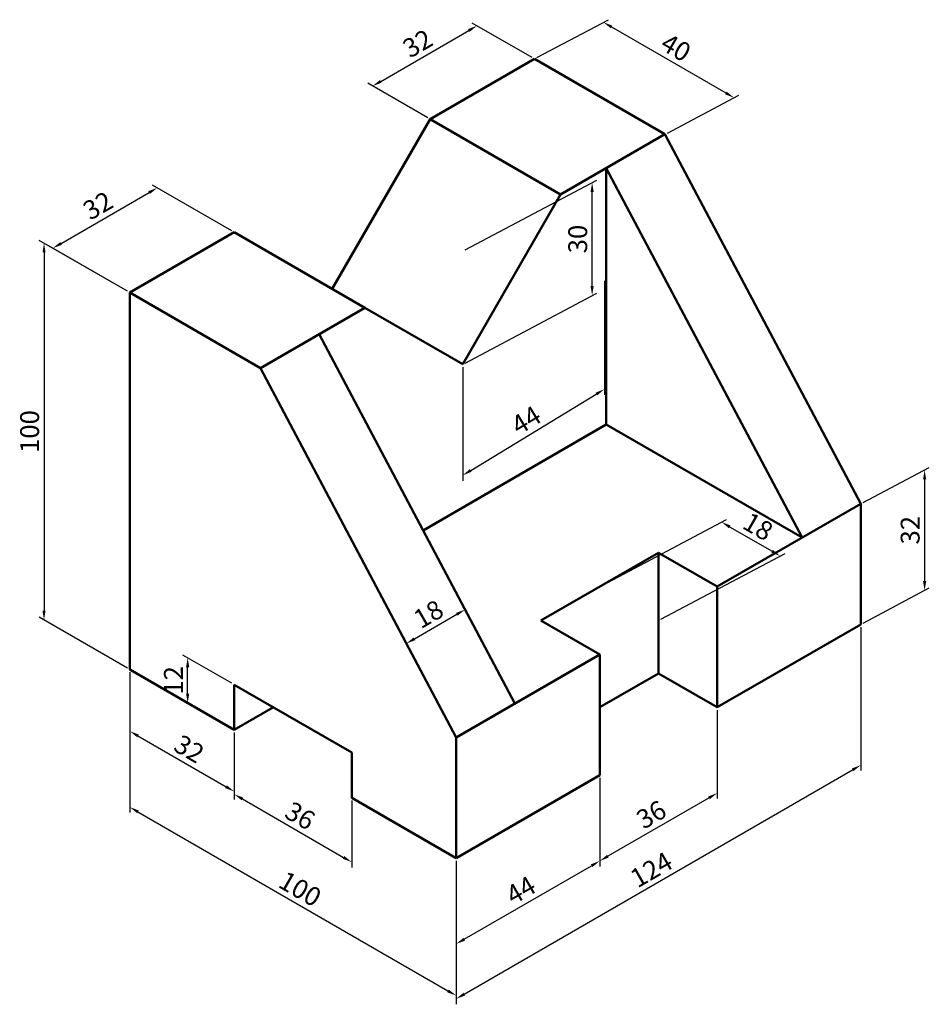
# Model space of a CAD drawing. Units: millimetres. Extents: x 91 to 333, y -17 to 244.
import ezdxf

# ---------------------------------------------------------------- set-up
doc = ezdxf.new("R2010")
doc.units = ezdxf.units.MM
doc.layers.add('M-DIMS', color=2, linetype='Continuous', lineweight=25)
doc.layers.add('M-OUTL', color=7, linetype='Continuous', lineweight=50)
doc.styles.get("Standard").update_dxf_attribs({"font": 'arial.ttf'})
doc.dimstyles.new('ISO-25', dxfattribs={"dimtxt": 5, "dimasz": 2.5, "dimexe": 1.25, "dimexo": 0.625, "dimtad": 1, "dimtxsty": 'Standard', "dimcen": 2.5, "dimadec": 0, "dimazin": 0, "dimtfac": 1, "dimtmove": 0, "dimatfit": 3, "dimfxl": 1, "dimarcsym": 0})

# ---------------------------------------------------------------- blocks, each defined once
blk = doc.blocks.new('*D1')
at = {"layer": 'Defpoints', "color": 0, "transparency": 16777216}
for p in [(127.79, 199.74), (148.21, 187.94), (120.5, 171.94)]:
    blk.add_point(p, dxfattribs=at)
at = {"layer": 'M-DIMS', "color": 0, "lineweight": -2, "transparency": 16777216}
for p, q in [((147.59, 188.3), (126.54, 200.46)), ((102.24, 184.99), (125.62, 198.49)), ((119.88, 172.3), (98.82, 184.46))]:
    blk.add_line(p, q, dxfattribs=at)
at = {"layer": 'M-DIMS', "color": 0, "transparency": 16777216}
for points in [[(125.41, 198.85), (125.83, 198.13), (127.79, 199.74)], [(102.03, 185.35), (102.45, 184.63), (100.07, 183.74)]]:
    blk.add_solid(points, dxfattribs=at)
at = {"layer": 'M-DIMS', "color": 0, "transparency": 16777216, "insert": (112.34, 194.49), "char_height": 5, "attachment_point": 5, "rotation": 30}
blk.add_mtext('32', dxfattribs=at)
blk = doc.blocks.new('*D2')
at = {"layer": 'Defpoints', "color": 0, "transparency": 16777216}
for p in [(227.89, 233.94), (280.85, 223.66), (262.53, 213.94)]:
    blk.add_point(p, dxfattribs=at)
at = {"layer": 'M-DIMS', "color": 0, "lineweight": -2, "transparency": 16777216}
for p, q in [((228.54, 234.29), (247.51, 244.35)), ((248.37, 242.41), (278.68, 224.91)), ((263.18, 214.29), (282.15, 224.35))]:
    blk.add_line(p, q, dxfattribs=at)
at = {"layer": 'M-DIMS', "color": 0, "transparency": 16777216}
for points in [[(248.58, 242.77), (248.17, 242.05), (246.21, 243.66)], [(278.89, 225.27), (278.48, 224.55), (280.85, 223.66)]]:
    blk.add_solid(points, dxfattribs=at)
at = {"layer": 'M-DIMS', "color": 0, "transparency": 16777216, "insert": (265.12, 236.41), "char_height": 5, "attachment_point": 5, "rotation": 330}
blk.add_mtext('40', dxfattribs=at)
blk = doc.blocks.new('*D3')
at = {"layer": 'Defpoints', "color": 0, "transparency": 16777216}
for p in [(120.5, 171.94), (97.73, 85.09), (120.5, 71.94)]:
    blk.add_point(p, dxfattribs=at)
at = {"layer": 'M-DIMS', "color": 0, "lineweight": -2, "transparency": 16777216}
for p, q in [((119.88, 172.3), (96.48, 185.81)), ((97.73, 182.59), (97.73, 87.59)), ((119.88, 72.3), (96.48, 85.81))]:
    blk.add_line(p, q, dxfattribs=at)
at = {"layer": 'M-DIMS', "color": 0, "transparency": 16777216}
for points in [[(97.32, 182.59), (98.15, 182.59), (97.73, 185.09)], [(97.32, 87.59), (98.15, 87.59), (97.73, 85.09)]]:
    blk.add_solid(points, dxfattribs=at)
at = {"layer": 'M-DIMS', "color": 0, "transparency": 16777216, "insert": (94.56, 135.09), "char_height": 5, "attachment_point": 5, "rotation": 90}
blk.add_mtext('100', dxfattribs=at)
blk = doc.blocks.new('*D4')
at = {"layer": 'Defpoints', "color": 0, "transparency": 16777216}
for p in [(209.48, 87.87), (222.69, 62.94), (207.1, 53.94)]:
    blk.add_point(p, dxfattribs=at)
at = {"layer": 'M-DIMS', "color": 0, "lineweight": -2, "transparency": 16777216}
for p, q in [((222.4, 63.5), (208.89, 88.97)), ((196.05, 80.12), (207.31, 86.62)), ((206.81, 54.5), (193.3, 79.97))]:
    blk.add_line(p, q, dxfattribs=at)
at = {"layer": 'M-DIMS', "color": 0, "transparency": 16777216}
for points in [[(207.1, 86.98), (207.52, 86.26), (209.48, 87.87)], [(195.85, 80.48), (196.26, 79.76), (193.89, 78.87)]]:
    blk.add_solid(points, dxfattribs=at)
at = {"layer": 'M-DIMS', "color": 0, "transparency": 16777216, "insert": (200.09, 86.12), "char_height": 5, "attachment_point": 5, "rotation": 30}
blk.add_mtext('18', dxfattribs=at)
blk = doc.blocks.new('*D5')
at = {"layer": 'Defpoints', "color": 0, "transparency": 16777216}
for p in [(120.5, 71.94), (148.21, 55.94), (148.21, 39.61)]:
    blk.add_point(p, dxfattribs=at)
at = {"layer": 'M-DIMS', "color": 0, "lineweight": -2, "transparency": 16777216}
for p, q in [((120.5, 71.22), (120.5, 54.17)), ((148.21, 55.22), (148.21, 38.17)), ((122.67, 54.36), (146.05, 40.86))]:
    blk.add_line(p, q, dxfattribs=at)
at = {"layer": 'M-DIMS', "color": 0, "transparency": 16777216}
for points in [[(122.87, 54.72), (122.46, 54), (120.5, 55.61)], [(146.26, 41.22), (145.84, 40.5), (148.21, 39.61)]]:
    blk.add_solid(points, dxfattribs=at)
at = {"layer": 'M-DIMS', "color": 0, "transparency": 16777216, "insert": (135.95, 50.36), "char_height": 5, "attachment_point": 5, "rotation": 330}
blk.add_mtext('32', dxfattribs=at)
blk = doc.blocks.new('*D6')
at = {"layer": 'Defpoints', "color": 0, "transparency": 16777216}
for p in [(135.85, 75.08), (148.21, 67.94), (148.21, 55.94)]:
    blk.add_point(p, dxfattribs=at)
at = {"layer": 'M-DIMS', "color": 0, "lineweight": -2, "transparency": 16777216}
for p, q in [((147.59, 68.3), (134.6, 75.8)), ((135.85, 65.58), (135.85, 72.58)), ((147.59, 56.3), (134.6, 63.8))]:
    blk.add_line(p, q, dxfattribs=at)
at = {"layer": 'M-DIMS', "color": 0, "transparency": 16777216}
for points in [[(135.44, 72.58), (136.27, 72.58), (135.85, 75.08)], [(135.44, 65.58), (136.27, 65.58), (135.85, 63.08)]]:
    blk.add_solid(points, dxfattribs=at)
at = {"layer": 'M-DIMS', "color": 0, "transparency": 16777216, "insert": (132.72, 69.08), "char_height": 5, "attachment_point": 5, "rotation": 90}
blk.add_mtext('12', dxfattribs=at)
blk = doc.blocks.new('*D7')
at = {"layer": 'Defpoints', "color": 0, "transparency": 16777216}
for p in [(148.21, 55.94), (179.39, 37.94), (179.39, 20.88)]:
    blk.add_point(p, dxfattribs=at)
at = {"layer": 'M-DIMS', "color": 0, "lineweight": -2, "transparency": 16777216}
for p, q in [((148.21, 55.22), (148.21, 37.44)), ((150.38, 37.63), (177.23, 22.13)), ((179.39, 37.22), (179.39, 19.44))]:
    blk.add_line(p, q, dxfattribs=at)
at = {"layer": 'M-DIMS', "color": 0, "transparency": 16777216}
for points in [[(150.59, 37.99), (150.17, 37.27), (148.21, 38.88)], [(177.43, 22.49), (177.02, 21.77), (179.39, 20.88)]]:
    blk.add_solid(points, dxfattribs=at)
at = {"layer": 'M-DIMS', "color": 0, "transparency": 16777216, "insert": (165.39, 32.63), "char_height": 5, "attachment_point": 5, "rotation": 330}
blk.add_mtext('36', dxfattribs=at)
blk = doc.blocks.new('*D8')
at = {"layer": 'Defpoints', "color": 0, "transparency": 16777216}
for p in [(120.5, 71.94), (207.1, 21.94), (207.1, -14.54)]:
    blk.add_point(p, dxfattribs=at)
at = {"layer": 'M-DIMS', "color": 0, "lineweight": -2, "transparency": 16777216}
for p, q in [((120.5, 71.22), (120.5, 34.01)), ((122.67, 34.21), (204.94, -13.29)), ((207.1, 21.22), (207.1, -15.99))]:
    blk.add_line(p, q, dxfattribs=at)
at = {"layer": 'M-DIMS', "color": 0, "transparency": 16777216}
for points in [[(122.87, 34.57), (122.46, 33.85), (120.5, 35.46)], [(205.15, -12.93), (204.73, -13.65), (207.1, -14.54)]]:
    blk.add_solid(points, dxfattribs=at)
at = {"layer": 'M-DIMS', "color": 0, "transparency": 16777216, "insert": (165.39, 13.21), "char_height": 5, "attachment_point": 5, "rotation": 330}
blk.add_mtext('100', dxfattribs=at)
blk = doc.blocks.new('*D9')
at = {"layer": 'Defpoints', "color": 0, "transparency": 16777216}
for p in [(245.21, 43.94), (207.1, 21.94), (245.21, 21.17)]:
    blk.add_point(p, dxfattribs=at)
at = {"layer": 'M-DIMS', "color": 0, "lineweight": -2, "transparency": 16777216}
for p, q in [((245.21, 43.22), (245.21, 19.73)), ((207.1, 21.22), (207.1, -2.27)), ((209.27, 0.42), (243.04, 19.92))]:
    blk.add_line(p, q, dxfattribs=at)
at = {"layer": 'M-DIMS', "color": 0, "transparency": 16777216}
for points in [[(242.84, 20.28), (243.25, 19.56), (245.21, 21.17)], [(209.06, 0.78), (209.48, 0.06), (207.1, -0.83)]]:
    blk.add_solid(points, dxfattribs=at)
at = {"layer": 'M-DIMS', "color": 0, "transparency": 16777216, "insert": (224.59, 12.88), "char_height": 5, "attachment_point": 5, "rotation": 30}
blk.add_mtext('44', dxfattribs=at)
blk = doc.blocks.new('*D10')
at = {"layer": 'Defpoints', "color": 0, "transparency": 16777216}
for p in [(276.39, 61.94), (245.21, 43.94), (245.21, 21.18)]:
    blk.add_point(p, dxfattribs=at)
at = {"layer": 'M-DIMS', "color": 0, "lineweight": -2, "transparency": 16777216}
for p, q in [((276.39, 61.22), (276.39, 37.74)), ((245.21, 43.22), (245.21, 19.74)), ((274.22, 37.93), (247.37, 22.43))]:
    blk.add_line(p, q, dxfattribs=at)
at = {"layer": 'M-DIMS', "color": 0, "transparency": 16777216}
for points in [[(274.01, 38.29), (274.43, 37.57), (276.39, 39.18)], [(247.17, 22.79), (247.58, 22.07), (245.21, 21.18)]]:
    blk.add_solid(points, dxfattribs=at)
at = {"layer": 'M-DIMS', "color": 0, "transparency": 16777216, "insert": (259.21, 32.94), "char_height": 5, "attachment_point": 5, "rotation": 30}
blk.add_mtext('36', dxfattribs=at)
blk = doc.blocks.new('*D11')
at = {"layer": 'Defpoints', "color": 0, "transparency": 16777216}
for p in [(314.49, 83.94), (314.49, 46.6), (207.1, 21.94)]:
    blk.add_point(p, dxfattribs=at)
at = {"layer": 'M-DIMS', "color": 0, "lineweight": -2, "transparency": 16777216}
for p, q in [((314.49, 83.22), (314.49, 45.15)), ((209.27, -14.15), (312.33, 45.35)), ((207.1, 21.22), (207.1, -16.85))]:
    blk.add_line(p, q, dxfattribs=at)
at = {"layer": 'M-DIMS', "color": 0, "transparency": 16777216}
for points in [[(312.12, 45.71), (312.53, 44.99), (314.49, 46.6)], [(209.06, -13.79), (209.48, -14.51), (207.1, -15.4)]]:
    blk.add_solid(points, dxfattribs=at)
at = {"layer": 'M-DIMS', "color": 0, "transparency": 16777216, "insert": (259.23, 18.31), "char_height": 5, "attachment_point": 5, "rotation": 30}
blk.add_mtext('124', dxfattribs=at)
blk = doc.blocks.new('*D12')
at = {"layer": 'Defpoints', "color": 0, "transparency": 16777216}
for p in [(314.49, 115.94), (331.43, 92.92), (314.49, 83.94)]:
    blk.add_point(p, dxfattribs=at)
at = {"layer": 'M-DIMS', "color": 0, "lineweight": -2, "transparency": 16777216}
for p, q in [((315.12, 116.27), (332.68, 125.59)), ((331.43, 122.42), (331.43, 95.42)), ((315.12, 84.27), (332.68, 93.59))]:
    blk.add_line(p, q, dxfattribs=at)
at = {"layer": 'M-DIMS', "color": 0, "transparency": 16777216}
for points in [[(331.01, 122.42), (331.85, 122.42), (331.43, 124.92)], [(331.01, 95.42), (331.85, 95.42), (331.43, 92.92)]]:
    blk.add_solid(points, dxfattribs=at)
at = {"layer": 'M-DIMS', "color": 0, "transparency": 16777216, "insert": (328.25, 108.92), "char_height": 5, "attachment_point": 5, "rotation": 90}
blk.add_mtext('32', dxfattribs=at)
blk = doc.blocks.new('*D13')
at = {"layer": 'Defpoints', "color": 0, "transparency": 16777216}
for p in [(293.11, 102.08), (245.21, 93.94), (260.8, 84.94)]:
    blk.add_point(p, dxfattribs=at)
at = {"layer": 'M-DIMS', "color": 0, "lineweight": -2, "transparency": 16777216}
for p, q in [((245.86, 94.29), (278.83, 111.77)), ((279.69, 109.83), (290.95, 103.33)), ((261.45, 85.29), (294.42, 102.77))]:
    blk.add_line(p, q, dxfattribs=at)
at = {"layer": 'M-DIMS', "color": 0, "transparency": 16777216}
for points in [[(279.9, 110.19), (279.48, 109.47), (277.53, 111.08)], [(291.16, 103.69), (290.74, 102.97), (293.11, 102.08)]]:
    blk.add_solid(points, dxfattribs=at)
at = {"layer": 'M-DIMS', "color": 0, "transparency": 16777216, "insert": (286.91, 109.33), "char_height": 5, "attachment_point": 5, "rotation": 330}
blk.add_mtext('18', dxfattribs=at)
blk = doc.blocks.new('*D14')
at = {"layer": 'Defpoints', "color": 0, "transparency": 16777216}
for p in [(243.2, 201.16), (208.84, 182.94), (208.84, 152.94)]:
    blk.add_point(p, dxfattribs=at)
at = {"layer": 'M-DIMS', "color": 0, "lineweight": -2, "transparency": 16777216}
for p, q in [((209.46, 183.27), (244.45, 201.82)), ((243.2, 173.66), (243.2, 198.66)), ((209.46, 153.27), (244.45, 171.82))]:
    blk.add_line(p, q, dxfattribs=at)
at = {"layer": 'M-DIMS', "color": 0, "transparency": 16777216}
for points in [[(242.78, 198.66), (243.61, 198.66), (243.2, 201.16)], [(242.78, 173.66), (243.61, 173.66), (243.2, 171.16)]]:
    blk.add_solid(points, dxfattribs=at)
at = {"layer": 'M-DIMS', "color": 0, "transparency": 16777216, "insert": (240.02, 186.16), "char_height": 5, "attachment_point": 5, "rotation": 90}
blk.add_mtext('30', dxfattribs=at)
blk = doc.blocks.new('*D15')
at = {"layer": 'Defpoints', "color": 0, "transparency": 16777216}
for p in [(212.65, 242.74), (227.89, 233.94), (200.18, 217.94)]:
    blk.add_point(p, dxfattribs=at)
at = {"layer": 'M-DIMS', "color": 0, "lineweight": -2, "transparency": 16777216}
for p, q in [((227.26, 234.3), (211.4, 243.47)), ((187.1, 227.99), (210.48, 241.49)), ((199.55, 218.3), (183.68, 227.47))]:
    blk.add_line(p, q, dxfattribs=at)
at = {"layer": 'M-DIMS', "color": 0, "transparency": 16777216}
for points in [[(210.27, 241.85), (210.69, 241.13), (212.65, 242.74)], [(186.89, 228.35), (187.31, 227.63), (184.93, 226.74)]]:
    blk.add_solid(points, dxfattribs=at)
at = {"layer": 'M-DIMS', "color": 0, "transparency": 16777216, "insert": (197.2, 237.5), "char_height": 5, "attachment_point": 5, "rotation": 30}
blk.add_mtext('32', dxfattribs=at)
blk = doc.blocks.new('*D16')
at = {"layer": 'Defpoints', "color": 0, "transparency": 16777216}
for p in [(246.44, 175.8), (208.84, 152.94), (246.44, 146.32)]:
    blk.add_point(p, dxfattribs=at)
at = {"layer": 'M-DIMS', "color": 0, "lineweight": -2, "transparency": 16777216}
for p, q in [((246.44, 175.07), (246.44, 144.86)), ((208.84, 152.21), (208.84, 122.01)), ((210.97, 124.77), (244.3, 145.02))]:
    blk.add_line(p, q, dxfattribs=at)
at = {"layer": 'M-DIMS', "color": 0, "transparency": 16777216}
for points in [[(244.08, 145.38), (244.52, 144.67), (246.44, 146.32)], [(210.76, 125.12), (211.19, 124.41), (208.84, 123.47)]]:
    blk.add_solid(points, dxfattribs=at)
at = {"layer": 'M-DIMS', "color": 0, "transparency": 16777216, "insert": (226.01, 137.57), "char_height": 5, "attachment_point": 5, "rotation": 31.2909}
blk.add_mtext('44', dxfattribs=at)

msp = doc.modelspace()

# ---------------------------------------------------------------- linework, layer by layer
at = {"layer": 'M-OUTL'}
for p, q in [((200.175, 217.944), (227.888, 233.944)), ((227.888, 233.944), (262.529, 213.944)), ((174.195, 172.944), (200.175, 217.944)), ((200.175, 217.944), (234.816, 197.944)), ((262.529, 213.944), (234.816, 197.944)), ((262.529, 213.944), (314.491, 115.944)), ((246.941, 204.944), (298.902, 106.944)), ((246.941, 204.944), (246.941, 136.944)), ((208.836, 152.944), (234.816, 197.944)), ((148.214, 187.944), (120.501, 171.944)), ((182.855, 167.944), (148.214, 187.944)), ((120.501, 71.944), (120.501, 171.944)), ((120.501, 171.944), (155.142, 151.944)), ((155.142, 151.944), (182.855, 167.944)), ((208.836, 152.944), (182.855, 167.944)), ((170.731, 160.944), (222.692, 62.944)), ((155.142, 151.944), (207.104, 53.944)), ((246.941, 136.944), (198.335, 108.881)), ((298.902, 106.944), (246.941, 136.944)), ((276.386, 93.944), (314.491, 115.944)), ((314.491, 115.944), (314.491, 83.944)), ((229.62, 84.944), (260.797, 102.944)), ((276.386, 93.944), (260.797, 102.944)), ((260.797, 70.944), (260.797, 102.944)), ((276.386, 61.944), (276.386, 93.944)), ((245.209, 75.944), (229.62, 84.944)), ((314.491, 83.944), (276.386, 61.944)), ((207.104, 53.944), (245.209, 75.944)), ((245.209, 75.944), (245.209, 43.944)), ((120.501, 71.944), (148.214, 55.944)), ((245.209, 61.944), (260.797, 70.944)), ((276.386, 61.944), (260.797, 70.944)), ((148.214, 55.944), (148.214, 67.944)), ((148.214, 67.944), (179.391, 49.944)), ((148.214, 55.944), (158.606, 61.944)), ((207.104, 21.944), (207.104, 53.944)), ((179.391, 49.944), (179.391, 37.944)), ((245.209, 43.944), (207.104, 21.944)), ((179.391, 37.944), (207.104, 21.944))]:
    msp.add_line(p, q, dxfattribs=at)

# ---------------------------------------------------------------- dimensions: what is measured, and where the dimension line sits
at = {"layer": 'M-DIMS'}
for p1, p2, distance, picture, middle in [((200.175, 217.944), (227.888, 233.944), 15.242, '*D15', (197.2, 237.497)), ((227.888, 233.944), (262.529, 213.944), 17.573, '*D2', (265.118, 236.41)), ((208.836, 152.944), (208.836, 182.944), -34.36, '*D14', (240.016, 186.162)), ((120.501, 171.944), (148.214, 187.944), 20.428, '*D1', (112.339, 194.491)), ((120.501, 171.944), (120.501, 71.944), -22.768, '*D3', (94.555, 135.089)), ((208.836, 152.944), (246.436, 175.796), -25.187, '*D16', (226.013, 137.566)), ((314.491, 115.944), (314.491, 83.944), 16.938, '*D12', (328.249, 108.924)), ((245.209, 93.944), (260.797, 84.944), 30.998, '*D13', (286.909, 109.331)), ((207.104, 53.944), (222.692, 62.944), 28.193, '*D4', (200.094, 86.12)), ((207.104, 21.944), (314.491, 83.944), -32.344, '*D11', (259.23, 18.311)), ((148.214, 55.944), (148.214, 67.944), 12.36, '*D6', (132.718, 69.08)), ((120.501, 71.944), (148.214, 55.944), -14.146, '*D5', (135.947, 50.362)), ((120.501, 71.944), (207.104, 21.944), -31.599, '*D8', (165.391, 13.209)), ((276.386, 61.944), (245.209, 43.944), 19.712, '*D10', (259.207, 32.935)), ((148.214, 55.944), (179.391, 37.944), -14.778, '*D7', (165.392, 32.633)), ((207.104, 21.944), (245.209, 43.944), -19.722, '*D9', (224.594, 12.877))]:
    dim = msp.add_aligned_dim(p1=p1, p2=p2, distance=distance, dimstyle='ISO-25', override={"dimclrd": 0, "dimclre": 0, "dimclrt": 0}, dxfattribs=at)
    dim.commit()
    dim.dimension.update_dxf_attribs({"geometry": picture, "text_midpoint": middle})

doc.saveas('drawing.dxf')
